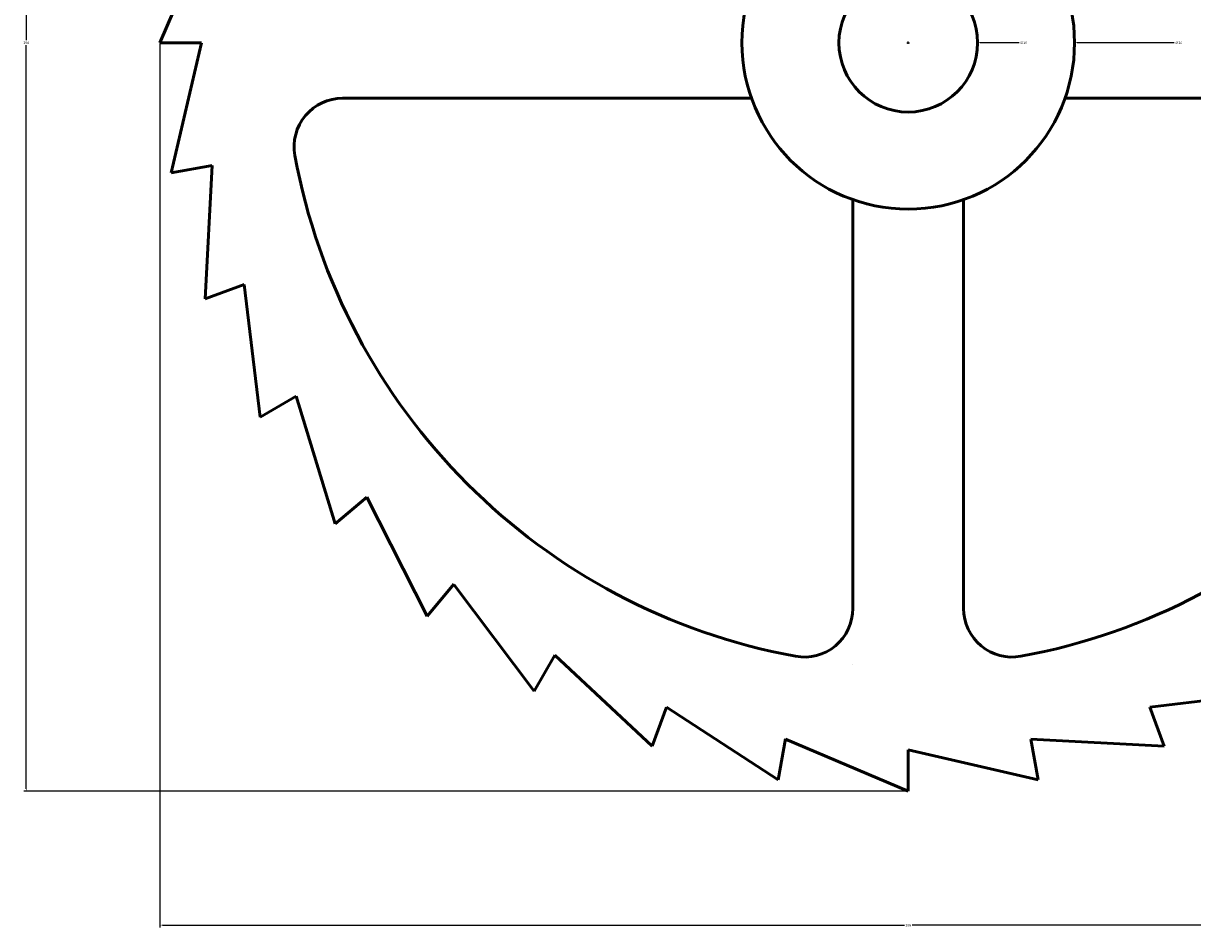
# Model space of a CAD drawing. Units: millimetres. Extents: x 3287 to 3415, y 1573 to 1701.
# Tile 1 of 3: x 3287 to 3371, y 1573 to 1639. Entities that reach past the tile are written whole.
import ezdxf

# ---------------------------------------------------------------- set-up
doc = ezdxf.new("R2010")
doc.units = ezdxf.units.MM
for name, color, linetype, lineweight in [('M-CONS', 8, 'Continuous', 18), ('M-DIMS', 2, 'Continuous', 18), ('M-OUTL', 7, 'Continuous', 50)]:
    doc.layers.add(name, color=color, linetype=linetype, lineweight=lineweight)
doc.styles.get("Standard").update_dxf_attribs({"font": 'arial.ttf'})
doc.dimstyles.get("Standard").update_dxf_attribs({"dimtxt": 0.18, "dimasz": 0.18, "dimexe": 0.18, "dimexo": 0.0625, "dimgap": 0.09, "dimtad": 0, "dimtih": 1, "dimtoh": 1, "dimdec": 4, "dimzin": 0, "dimdsep": 46, "dimtxsty": 'Standard', "dimcen": 0.09, "dimadec": 0, "dimazin": 0, "dimtfac": 1, "dimtdec": 4, "dimtofl": 0, "dimtmove": 0, "dimatfit": 3, "dimfxl": 1, "dimtolj": 1, "dimtzin": 0, "dimarcsym": 0})

# ---------------------------------------------------------------- blocks, each defined once
blk = doc.blocks.new('RATCHET-TOOTH-10DEG')
for p, q in [((0, 8.856), (2.954, 9.377)), ((2.954, 9.377), (0.775, 0))]:
    blk.add_line(p, q)
blk = doc.blocks.new('WHEEL-SPOKE-OPENING')
for points in [[(40.317, 7.314), (40.317, 36.817)], [(3.5, 0), (33.003, 0)]]:
    blk.add_lwpolyline(points)
for centre, radius, start, end in [((44.317, -4), 45, 100.41187, 169.58813), ((36.817, 36.817), 3.5, 0, 100.41187), ((3.5, 3.5), 3.5, 169.58813, 270)]:
    blk.add_arc(centre, radius, start, end)
blk = doc.blocks.new('*D3')
at = {"layer": 'Defpoints', "color": 0, "transparency": 16777216}
for p in [(3296.972, 1637.286), (3404.972, 1637.286), (3404.972, 1573.636)]:
    blk.add_point(p, dxfattribs=at)
at = {"layer": 'M-DIMS', "color": 0, "lineweight": -2, "transparency": 16777216}
for p, q in [((3296.972, 1637.224), (3296.972, 1573.456)), ((3404.972, 1637.224), (3404.972, 1573.456)), ((3297.152, 1573.636), (3350.691, 1573.636)), ((3404.792, 1573.636), (3351.252, 1573.636))]:
    blk.add_line(p, q, dxfattribs=at)
at = {"layer": 'M-DIMS', "color": 0, "transparency": 16777216}
for points in [[(3297.152, 1573.666), (3297.152, 1573.606), (3296.972, 1573.636)], [(3404.792, 1573.666), (3404.792, 1573.606), (3404.972, 1573.636)]]:
    blk.add_solid(points, dxfattribs=at)
at = {"layer": 'M-DIMS', "color": 0, "transparency": 16777216, "insert": (3350.972, 1573.636), "char_height": 0.18, "attachment_point": 5}
blk.add_mtext('\\A1;108', dxfattribs=at)
blk = doc.blocks.new('*D4')
at = {"layer": 'Defpoints', "color": 0, "transparency": 16777216}
for p in [(3287.322, 1691.286), (3350.972, 1691.286), (3350.972, 1583.286)]:
    blk.add_point(p, dxfattribs=at)
at = {"layer": 'M-DIMS', "color": 0, "lineweight": -2, "transparency": 16777216}
for p, q in [((3350.909, 1691.286), (3287.142, 1691.286)), ((3287.322, 1691.106), (3287.322, 1637.468)), ((3287.322, 1583.466), (3287.322, 1637.104)), ((3350.909, 1583.286), (3287.142, 1583.286))]:
    blk.add_line(p, q, dxfattribs=at)
at = {"layer": 'M-DIMS', "color": 0, "transparency": 16777216}
for points in [[(3287.292, 1691.106), (3287.352, 1691.106), (3287.322, 1691.286)], [(3287.292, 1583.466), (3287.352, 1583.466), (3287.322, 1583.286)]]:
    blk.add_solid(points, dxfattribs=at)
at = {"layer": 'M-DIMS', "color": 0, "transparency": 16777216, "insert": (3287.322, 1637.286), "char_height": 0.18, "attachment_point": 5}
blk.add_mtext('\\A1;108', dxfattribs=at)
blk = doc.blocks.new('*D7')
at = {"layer": 'Defpoints', "color": 0, "transparency": 16777216}
for p in [(3319.152, 1669.106), (3350.972, 1637.286)]:
    blk.add_point(p, dxfattribs=at)
at = {"layer": 'M-DIMS', "color": 0, "lineweight": -2, "transparency": 16777216}
for p, q in [((3299.88, 1688.198), (3300.06, 1688.198)), ((3300.06, 1688.198), (3319.025, 1669.233)), ((3350.882, 1637.286), (3351.062, 1637.286)), ((3350.972, 1637.196), (3350.972, 1637.376))]:
    blk.add_line(p, q, dxfattribs=at)
at = {"layer": 'M-DIMS', "color": 0, "transparency": 16777216}
blk.add_solid([(3319.046, 1669.254), (3319.004, 1669.212), (3319.152, 1669.106)], dxfattribs=at)
at = {"layer": 'M-DIMS', "color": 0, "transparency": 16777216, "insert": (3299.377, 1688.198), "char_height": 0.18, "attachment_point": 5}
blk.add_mtext('\\A1;4X R45', dxfattribs=at)
blk = doc.blocks.new('*D9')
at = {"layer": 'Defpoints', "color": 0, "transparency": 16777216}
for p in [(3338.972, 1637.286), (3362.972, 1637.286)]:
    blk.add_point(p, dxfattribs=at)
at = {"layer": 'M-DIMS', "color": 0, "lineweight": -2, "transparency": 16777216}
for p, q in [((3350.882, 1637.286), (3351.062, 1637.286)), ((3350.972, 1637.196), (3350.972, 1637.376)), ((3370.172, 1637.286), (3363.152, 1637.286))]:
    blk.add_line(p, q, dxfattribs=at)
at = {"layer": 'M-DIMS', "color": 0, "transparency": 16777216}
blk.add_solid([(3363.152, 1637.316), (3363.152, 1637.256), (3362.972, 1637.286)], dxfattribs=at)
at = {"layer": 'M-DIMS', "color": 0, "transparency": 16777216, "insert": (3370.488, 1637.286), "char_height": 0.18, "attachment_point": 5}
blk.add_mtext('\\A1;∅24', dxfattribs=at)
blk = doc.blocks.new('*D10')
at = {"layer": 'Defpoints', "color": 0, "transparency": 16777216}
for p in [(3345.972, 1637.286), (3355.972, 1637.286)]:
    blk.add_point(p, dxfattribs=at)
at = {"layer": 'M-DIMS', "color": 0, "lineweight": -2, "transparency": 16777216}
for p, q in [((3350.882, 1637.286), (3351.062, 1637.286)), ((3350.972, 1637.196), (3350.972, 1637.376)), ((3358.972, 1637.286), (3356.152, 1637.286))]:
    blk.add_line(p, q, dxfattribs=at)
at = {"layer": 'M-DIMS', "color": 0, "transparency": 16777216}
blk.add_solid([(3356.152, 1637.316), (3356.152, 1637.256), (3355.972, 1637.286)], dxfattribs=at)
at = {"layer": 'M-DIMS', "color": 0, "transparency": 16777216, "insert": (3359.288, 1637.286), "char_height": 0.18, "attachment_point": 5}
blk.add_mtext('\\A1;∅10', dxfattribs=at)

msp = doc.modelspace()

# ---------------------------------------------------------------- linework, layer by layer
at = {"layer": 'M-CONS'}
msp.add_lwpolyline([(3346.972, 1592.464), (3346.972, 1592.464)], close=True, dxfattribs=at)
at = {"layer": 'M-OUTL'}
for radius in [12, 5]:
    msp.add_circle((3350.972, 1637.286), radius, dxfattribs=at)

# ---------------------------------------------------------------- block references
for name, p, rotation in [('RATCHET-TOOTH-10DEG', (3301.509, 1646.008), 169.9999999999888), ('RATCHET-TOOTH-10DEG', (3300.746, 1637.286), 180), ('WHEEL-SPOKE-OPENING', (3346.972, 1592.969), 90.00000000000134), ('WHEEL-SPOKE-OPENING', (3395.288, 1633.286), 180), ('RATCHET-TOOTH-10DEG', (3301.509, 1628.565), 189.9999999999969), ('RATCHET-TOOTH-10DEG', (3303.775, 1620.108), 200), ('RATCHET-TOOTH-10DEG', (3307.475, 1612.173), 209.9999999999984), ('RATCHET-TOOTH-10DEG', (3312.497, 1605.002), 220.0000000000005), ('RATCHET-TOOTH-10DEG', (3318.687, 1598.811), 229.9999999999978), ('RATCHET-TOOTH-10DEG', (3325.859, 1593.79), 239.9999999999987), ('RATCHET-TOOTH-10DEG', (3368.15, 1590.09), 290.0000000000052), ('RATCHET-TOOTH-10DEG', (3333.794, 1590.09), 249.9999999999984), ('RATCHET-TOOTH-10DEG', (3359.693, 1587.824), 279.999999999997), ('RATCHET-TOOTH-10DEG', (3342.25, 1587.824), 260.0000000000052), ('RATCHET-TOOTH-10DEG', (3350.972, 1587.061), 270.0000000000019)]:
    msp.add_blockref(name, p, dxfattribs=dict(at, rotation=rotation))

# ---------------------------------------------------------------- dimensions: what is measured, and where the dimension line sits
at = {"layer": 'M-DIMS'}
dim = msp.add_linear_dim(base=(3287.322, 1691.286), p1=(3350.972, 1583.286), p2=(3350.972, 1691.286), angle=90, dimstyle='Standard', override={"dimdec": 0, "dimlfac": 1, "dimrnd": 0, "dimzin": 0, "dimdsep": 46, "dimlunit": 2}, dxfattribs=at)
dim.commit()
dim.dimension.update_dxf_attribs({"geometry": '*D4', "text_midpoint": (3287.322, 1637.286)})
dim = msp.add_radius_dim(center=(3350.972, 1637.286), mpoint=(3319.152, 1669.106), text='4X <>', dimstyle='Standard', override={"dimdec": 0, "dimlfac": 1, "dimrnd": 0, "dimzin": 0, "dimdsep": 46, "dimlunit": 2}, dxfattribs=at)
dim.commit()
dim.dimension.update_dxf_attribs({"geometry": '*D7', "text_midpoint": (3299.377, 1688.198), "dimtype": 164})
dim = msp.add_linear_dim(base=(3404.972, 1573.636), p1=(3296.972, 1637.286), p2=(3404.972, 1637.286), dimstyle='Standard', override={"dimdec": 0, "dimlfac": 1, "dimrnd": 0, "dimzin": 0, "dimdsep": 46, "dimlunit": 2}, dxfattribs=at)
dim.commit()
dim.dimension.update_dxf_attribs({"geometry": '*D3', "text_midpoint": (3350.972, 1573.636)})
for p1, p2, picture, middle in [((3338.972, 1637.286), (3362.972, 1637.286), '*D9', (3370.172, 1637.286)), ((3345.972, 1637.286), (3355.972, 1637.286), '*D10', (3358.972, 1637.286))]:
    dim = msp.add_diameter_dim_2p(p1=p1, p2=p2, dimstyle='Standard', override={"dimdec": 0, "dimlfac": 1, "dimrnd": 0, "dimzin": 0, "dimdsep": 46, "dimlunit": 2}, dxfattribs=at)
    dim.commit()
    dim.dimension.update_dxf_attribs({"geometry": picture, "text_midpoint": middle, "dimtype": 163})

doc.saveas('drawing.dxf')
